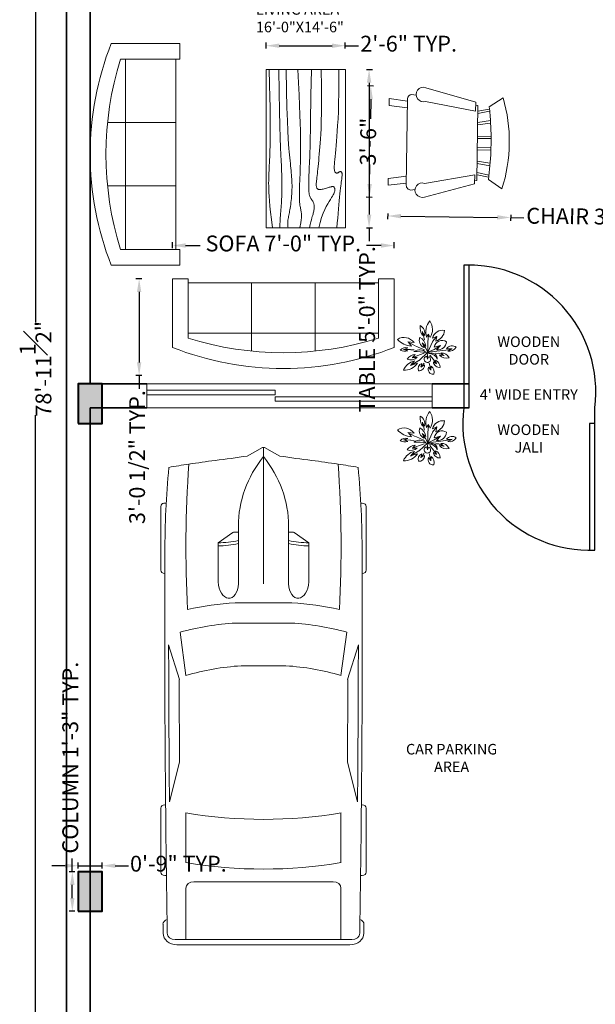
# Model space of a CAD drawing. Units: inches. Extents: x 2845 to 3575, y 808 to 1996.
# Tile 2 of 6: x 2955 to 3173, y 1215 to 1588. Entities that reach past the tile are written whole.
import ezdxf

# ---------------------------------------------------------------- set-up
doc = ezdxf.new("R2010")
doc.units = ezdxf.units.IN
for name, color, linetype, lineweight in [('A-ANNO-DIMS', 2, 'Continuous', 18), ('A-ANNO-TEXT', 7, 'Continuous', 18), ('A-AREA-IDEN', 7, 'Continuous', 18), ('A-COLS', 7, 'Continuous', 40), ('A-DOOR', 34, 'Continuous', 25), ('A-FURN', 30, 'Continuous', 18), ('A-GLAZ', 4, 'Continuous', 18), ('A-WALL', 1, 'Continuous', 35), ('C-PRKG-VEHI', 8, 'Continuous', 13), ('L-PLNT', 3, 'Continuous', 13)]:
    doc.layers.add(name, color=color, linetype=linetype, lineweight=lineweight)
doc.styles.get("Standard").update_dxf_attribs({"font": 'arial.ttf'})
doc.dimstyles.new('ISO-25', dxfattribs={"dimtxt": 6, "dimasz": 5, "dimexe": 1.25, "dimexo": 0.625, "dimtad": 0, "dimlunit": 4, "dimtxsty": 'Standard', "dimcen": 2.5, "dimclrd": 1, "dimclre": 1, "dimclrt": 1, "dimadec": 0, "dimazin": 0, "dimtfac": 1, "dimtmove": 0, "dimatfit": 3, "dimfxl": 1, "dimfxlon": 1, "dimfrac": 1, "dimarcsym": 0})

# ---------------------------------------------------------------- blocks, each defined once
blk = doc.blocks.new('Sofa - Roundback 7 ft.')
for p, q in [((-12.00002, -32.4421), (-12.00003, -6.5971)), ((11.99997, -32.4421), (11.99998, -6.5971)), ((-36.000027, -34), (-36.000027, -11.4696)), ((-35.999844, -13.3819), (35.9998, -13.3819)), ((35.99998, -34), (35.99998, -11.4696)), ((-36.000027, -32.4421), (35.99998, -32.4421))]:
    blk.add_line(p, q)
for points in [[(-36.000027, -34), (-42.000027, -34), (-42.000027, -8)], [(41.99998, -8), (41.99998, -34), (35.99998, -34)]]:
    blk.add_lwpolyline(points)
for centre, radius, start, end in [((0, -114.25), 114.25, 68.43141, 111.5686), ((-0.00001, -127.1968), 121.1968, 72.72033, 107.2797)]:
    blk.add_arc(centre, radius, start, end)
blk = doc.blocks.new('Table - Rectangular Woodgrain 60 x 30 in.')
for p, q in [((0, 0), (0, -30)), ((60, 0), (0, 0)), ((60, -30), (60, 0)), ((0, -30), (60, -30))]:
    blk.add_line(p, q)
for points in [[(0, -2.4), (4.8155, -2.418), (9.0302, -2.4688), (12.709, -2.5477), (15.9167, -2.65), (18.7181, -2.7711), (21.1781, -2.9063), (23.3616, -3.0508), (25.3333, -3.2), (27.1477, -3.3495), (28.8172, -3.4958), (30.3437, -3.636), (31.7291, -3.7667), (32.9756, -3.8849), (34.0849, -3.9875), (35.059, -4.0714), (35.9, -4.1334), (36.6114, -4.1711), (37.2041, -4.1854), (37.6906, -4.1779), (38.0833, -4.15), (38.3948, -4.1034), (38.6375, -4.0396), (38.8239, -3.9602), (38.9666, -3.8667), (39.0764, -3.7608), (39.1573, -3.6448), (39.2116, -3.521), (39.2416, -3.3917), (39.2498, -3.2593), (39.2385, -3.1261), (39.21, -2.9944), (39.1666, -2.8667), (39.111, -2.7447), (39.0468, -2.6281), (38.978, -2.5163), (38.9083, -2.4083), (38.8418, -2.3035), (38.7823, -2.201), (38.7337, -2.1001), (38.7, -2), (38.6844, -1.9003), (38.6875, -1.8021), (38.7094, -1.707), (38.75, -1.6167), (38.8094, -1.5326), (38.8875, -1.4563), (38.9844, -1.3893), (39.1, -1.3333), (39.2351, -1.2896), (39.3937, -1.2583), (39.5804, -1.2396), (39.8, -1.2333), (40.057, -1.2396), (40.3562, -1.2583), (40.7023, -1.2896), (41.1, -1.3333), (41.5547, -1.3895), (42.0755, -1.4573), (42.6721, -1.5361), (43.3542, -1.625), (44.1316, -1.7233), (45.014, -1.8302), (46.0114, -1.9449), (47.1333, -2.0667), (48.3862, -2.1947), (49.7625, -2.3281), (51.2513, -2.4663), (52.8416, -2.6083), (54.5226, -2.7535), (56.2833, -2.9011), (58.1127, -3.0501), (60, -3.2)], [(0, -9.2), (6.5759, -9.0858), (11.9385, -9.0365), (16.2527, -9.0418), (19.6833, -9.0917), (22.3952, -9.1759), (24.5531, -9.2844), (26.322, -9.4069), (27.8666, -9.5333), (29.3241, -9.6553), (30.7203, -9.7719), (32.0532, -9.8837), (33.3208, -9.9917), (34.5213, -10.0965), (35.6526, -10.199), (36.7128, -10.2999), (37.7, -10.4), (38.6129, -10.4996), (39.4531, -10.5969), (40.223, -10.6895), (40.925, -10.775), (41.5613, -10.8512), (42.1344, -10.9156), (42.6465, -10.966), (43.1, -11), (43.4976, -11.0158), (43.8437, -11.0136), (44.143, -10.9942), (44.4, -10.9583), (44.6195, -10.9069), (44.8062, -10.8406), (44.9648, -10.7603), (45.1, -10.6667), (45.2155, -10.5598), (45.3114, -10.4365), (45.3871, -10.2929), (45.4416, -10.125), (45.4743, -9.929), (45.4844, -9.7011), (45.4709, -9.4371), (45.4333, -9.1333), (45.3716, -8.7883), (45.2896, -8.4104), (45.1919, -8.0107), (45.0833, -7.6), (44.9685, -7.1893), (44.8521, -6.7896), (44.7388, -6.4117), (44.6333, -6.0667), (44.54, -5.7628), (44.4614, -5.4979), (44.4001, -5.2675), (44.3583, -5.0667), (44.3384, -4.8909), (44.3427, -4.7354), (44.3736, -4.5956), (44.4333, -4.4667), (44.5236, -4.3453), (44.6427, -4.2333), (44.7884, -4.1339), (44.9583, -4.05), (45.1501, -3.9849), (45.3614, -3.9417), (45.59, -3.9234), (45.8333, -3.9333), (46.0915, -3.9749), (46.3734, -4.0531), (46.6906, -4.1736), (47.0542, -4.3417), (47.4756, -4.5629), (47.9661, -4.8427), (48.5372, -5.1866), (49.2, -5.6), (49.9676, -6.0844), (50.8594, -6.625), (51.8965, -7.2031), (53.1, -7.8), (54.491, -8.3969), (56.0906, -8.975), (57.9199, -9.5156), (60, -10)], [(0, -12.8), (5.1847, -12.9322), (9.6213, -13.0323), (13.3963, -13.1059), (16.5958, -13.1583), (19.3063, -13.1952), (21.614, -13.2219), (23.6054, -13.2439), (25.3666, -13.2667), (26.9728, -13.2947), (28.4531, -13.3281), (29.8256, -13.3663), (31.1083, -13.4083), (32.3191, -13.4535), (33.476, -13.501), (34.597, -13.5501), (35.7, -13.6), (36.7984, -13.6497), (37.8875, -13.6979), (38.9578, -13.743), (40, -13.7833), (41.0047, -13.8174), (41.9625, -13.8438), (42.864, -13.8607), (43.7, -13.8667), (44.4631, -13.8604), (45.1552, -13.8417), (45.7801, -13.8104), (46.3416, -13.7667), (46.8439, -13.7104), (47.2906, -13.6417), (47.6858, -13.5604), (48.0333, -13.4667), (48.3375, -13.3608), (48.6042, -13.2448), (48.8396, -13.121), (49.05, -12.9917), (49.2417, -12.8593), (49.4208, -12.7261), (49.5937, -12.5944), (49.7667, -12.4667), (49.9452, -12.3451), (50.1323, -12.2313), (50.3303, -12.1268), (50.5416, -12.0333), (50.7686, -11.9524), (51.0135, -11.8854), (51.2788, -11.8341), (51.5666, -11.8), (51.8785, -11.7843), (52.2116, -11.7865), (52.562, -11.8059), (52.926, -11.8417), (53.2998, -11.8931), (53.6795, -11.9594), (54.0614, -12.0397), (54.4416, -12.1333), (54.8223, -12.2401), (55.2293, -12.3625), (55.6942, -12.5037), (56.2489, -12.6667), (56.9251, -12.8547), (57.7545, -13.0708), (58.7689, -13.3182), (60, -13.6)], [(0, -18), (5.124, -17.7273), (9.6609, -17.5057), (13.6705, -17.3303), (17.2125, -17.1958), (20.3467, -17.0973), (23.1328, -17.0297), (25.6307, -16.9878), (27.9, -16.9667), (29.9928, -16.9617), (31.9302, -16.9703), (33.7254, -16.9907), (35.3917, -17.0208), (36.9423, -17.0588), (38.3906, -17.1026), (39.7499, -17.1503), (41.0333, -17.2), (42.2519, -17.2496), (43.4073, -17.2969), (44.4986, -17.3395), (45.525, -17.375), (46.4858, -17.4012), (47.3802, -17.4156), (48.2074, -17.416), (48.9667, -17.4), (49.6583, -17.3662), (50.2872, -17.3167), (50.8595, -17.2547), (51.3812, -17.1833), (51.8584, -17.1057), (52.2971, -17.025), (52.7034, -16.9443), (53.0833, -16.8667), (53.443, -16.7951), (53.789, -16.7313), (54.128, -16.6768), (54.4666, -16.6334), (54.8115, -16.6024), (55.1693, -16.5854), (55.5465, -16.5841), (55.95, -16.6), (56.3828, -16.6337), (56.8346, -16.6823), (57.2915, -16.7418), (57.7396, -16.8084), (58.165, -16.878), (58.5539, -16.9469), (58.8924, -17.0111), (59.1666, -17.0667), (59.3679, -17.1107), (59.5078, -17.1438), (59.6032, -17.1675), (59.6708, -17.1833), (59.7275, -17.193), (59.7901, -17.1979), (59.8753, -17.1998), (60, -17.2)], [(0, -22.4), (8.0098, -22.2501), (14.4094, -22.1011), (19.4168, -21.9535), (23.25, -21.8083), (26.1269, -21.6663), (28.2656, -21.5281), (29.884, -21.3947), (31.2, -21.2667), (32.3967, -21.1448), (33.5172, -21.0292), (34.5697, -20.9198), (35.5625, -20.8167), (36.5037, -20.7198), (37.4015, -20.6292), (38.2642, -20.5448), (39.1, -20.4667), (39.9164, -20.3951), (40.7187, -20.3313), (41.5117, -20.2768), (42.3, -20.2333), (43.0883, -20.2024), (43.8812, -20.1854), (44.6836, -20.1841), (45.5, -20.2), (46.3328, -20.234), (47.1747, -20.2844), (48.0163, -20.3488), (48.8479, -20.425), (49.66, -20.5106), (50.4429, -20.6031), (51.1872, -20.7004), (51.8833, -20.8), (52.5246, -20.8999), (53.1166, -20.9995), (53.6681, -21.0983), (54.1875, -21.1958), (54.6834, -21.2919), (55.1646, -21.3859), (55.6394, -21.4777), (56.1167, -21.5667), (56.6028, -21.6515), (57.0961, -21.7266), (57.5929, -21.7852), (58.0896, -21.8208), (58.5823, -21.8268), (59.0674, -21.7964), (59.5412, -21.723), (60, -21.6)], [(0, -25.2), (8.6355, -25.0504), (15.7026, -24.9031), (21.4049, -24.7606), (25.9458, -24.625), (29.529, -24.4988), (32.3578, -24.3844), (34.6359, -24.284), (36.5667, -24.2), (38.3213, -24.1341), (39.9417, -24.0854), (41.437, -24.0523), (42.8167, -24.0333), (44.0901, -24.0268), (45.2667, -24.0313), (46.3557, -24.0451), (47.3667, -24.0667), (48.309, -24.0947), (49.1928, -24.1287), (50.0284, -24.168), (50.826, -24.2125), (51.5959, -24.2617), (52.3483, -24.3151), (53.0935, -24.3725), (53.8417, -24.4334), (54.6009, -24.497), (55.3699, -24.561), (56.1454, -24.6226), (56.9239, -24.6792), (57.7021, -24.7279), (58.4764, -24.7662), (59.2435, -24.7911), (60, -24.8)], [(0, -28.8), (5.6867, -28.6681), (10.45, -28.5698), (14.407, -28.5012), (17.675, -28.4584), (20.3711, -28.4374), (22.6125, -28.4344), (24.5164, -28.4455), (26.2, -28.4667), (27.762, -28.4947), (29.2276, -28.5281), (30.6033, -28.5663), (31.8958, -28.6084), (33.1118, -28.6535), (34.2578, -28.7011), (35.3405, -28.7501), (36.3666, -28.8), (37.3443, -28.8497), (38.288, -28.8974), (39.2137, -28.9412), (40.1375, -28.9792), (41.0753, -29.0093), (42.0432, -29.0297), (43.0572, -29.0384), (44.1333, -29.0333), (45.2936, -29.0114), (46.5843, -28.9641), (48.0579, -28.8816), (49.7666, -28.7542), (51.7629, -28.5721), (54.0989, -28.3255), (56.8272, -28.0048), (60, -27.6)]]:
    blk.add_lwpolyline(points)
blk = doc.blocks.new('Chair - Rocking')
for p, q in [((-8, -4.5), (-10, -1.5)), ((8, -4.5), (10, -1.5)), ((-4.5, -7), (-4.96674, -4.19951)), ((-4, -7), (-4.40532, -4.16272)), ((-1.5, -4.05012), (-1.5, -7)), ((-1, -7), (-1, -4.05012)), ((1, -7), (1, -4.04655)), ((1.5, -4.05012), (1.5, -7)), ((4, -7), (4.40187, -4.18694)), ((4.5, -7), (4.96761, -4.19437)), ((-7.5, -4.5), (-7, -7)), ((-6.5, -7), (-7.02225, -4.43)), ((6.5, -7), (7, -4.4057)), ((7.5, -4.5), (7, -7)), ((-9, -7.5), (-12, -18.49999)), ((-7, -7.5), (-9, -7.5)), ((-9, -18.49999), (-7, -7.5)), ((-8.23428, -6.99939), (-8.3093, -7.47958)), ((-8.23041, -7), (8.23915, -7)), ((7, -7.5), (9, -7.5)), ((9, -18.49999), (7, -7.5)), ((8.31071, -7.48854), (8.23449, -7.00073)), ((9, -7.5), (12, -18.49999)), ((-10.36644, -20.64523), (-10.5, -21.49999)), ((10.5, -21.49999), (10.3575, -20.58798)), ((-9, -22.49999), (-9.5, -26.49999)), ((0, -22.49999), (-9.5, -22.49999)), ((-8, -26.49999), (-7.5, -22.49999)), ((0, -22.49999), (9.5, -22.49999)), ((8, -26.49999), (7.5, -22.49999)), ((9, -22.49999), (9.5, -26.49999)), ((-9.5, -26.49999), (-8, -26.49999)), ((9.5, -26.49999), (8, -26.49999))]:
    blk.add_line(p, q)
for centre, radius, start, end in [((0, -34.08333), 34.08333, 72.93847, 107.0615), ((0, -68.25004), 64.25, 93.92211, 97.15267), ((0, -68.25004), 64.25, 82.84733, 93.92211), ((-10.5, -18.99999), 1.58114, 161.5651, 18.43495), ((10.5, -18.99999), 1.58114, 161.5651, 18.43495), ((-9.5, -21.49999), 1, 180, 270), ((9.5, -21.49999), 1, 270, 0)]:
    blk.add_arc(centre, radius, start, end)
blk = doc.blocks.new('z_109')
for p, q in [((-94, 294), (-122, 396)), ((-121, 393), (-119, 324)), ((-120, 377), (-82, 322)), ((-392, 202), (-278, 190)), ((-254, 128), (-392, 202)), ((-390, 202), (-327, 125)), ((-61, 92), (-128, 186)), ((-85, 244), (-94, 293)), ((-5, 350), (-42, 295)), ((-20, 11), (-18, 230)), ((-20, 11), (65, 205)), ((-14, 234), (-5, 350)), ((-5, 350), (24, 284)), ((65, 209), (150, 307)), ((65, 205), (65, 205)), ((150, 307), (68, 272)), ((129, 216), (150, 307)), ((150, 307), (129, 216)), ((-342, 60), (-472, 63)), ((-467, 63), (-392, 90)), ((-463, 64), (-392, 37)), ((-276, 53), (-338, 57)), ((-84, 54), (-246, 125)), ((-20, 11), (-181, -143)), ((-126, 184), (-60, 125)), ((-120, 176), (-91, 98)), ((-20, 11), (-61, 92)), ((-20, 11), (-24, -65)), ((-20, 11), (102, 64)), ((-20, 11), (-14, 11)), ((-14, 11), (319, 50)), ((-14, 11), (-13, 13)), ((-13, 13), (13, -13)), ((217, 135), (101, 105)), ((102, 64), (217, 135)), ((217, 135), (145, 55)), ((319, 50), (434, 75)), ((429, 74), (333, 77)), ((428, 74), (353, 32)), ((-187, -143), (-345, -240)), ((-342, -238), (-269, -151)), ((-178, -41), (-313, -92)), ((-308, -90), (-254, -33)), ((-306, -89), (-217, -88)), ((-86, -8), (-178, -41)), ((-26, -113), (-45, -66)), ((-24, -65), (-28, -121)), ((-28, -117), (-2, -69)), ((16, -43), (88, -126)), ((141, -208), (84, -170)), ((87, -129), (140, -204)), ((122, -8), (193, -11)), ((140, -205), (123, -139)), ((176, -10), (285, -54)), ((283, -54), (196, -42)), ((273, -52), (222, -4)), ((-328, -230), (-213, -195)), ((-151, -267), (-81, -228)), ((-89, -192), (-150, -267)), ((-150, -266), (-131, -199)), ((34, -320), (-6, -268)), ((4, -192), (16, -238)), ((16, -238), (35, -326)), ((35, -327), (45, -249))]:
    blk.add_line(p, q)
for centre, radius, start, end in [((262, 393), 319, 140.563, 197.8988), ((-221, 433), 288, 328.6458, 34.5329), ((84, 468), 249, 170.3029, 215.3262), ((-235, 368), 160, 343.2534, 62.5239), ((256, 231), 192, 77.7318, 167.6805), ((55, 447), 242, 287.7269, 353.3689), ((-464, 59), 228, 35.1725, 122.5976), ((-304, 504), 380, 221.8384, 266.6027), ((-21, 239), 158, 161.4501, 243.415), ((-251, 115), 192, 2.9136, 65.0019), ((247, 86), 147, 55.2824, 172.6291), ((167, 217), 164, 262.2896, 356.2544), ((-434, -39), 136, 71.6414, 139.5892), ((-450, 225), 197, 243.5199, 287.2599), ((-173, -118), 175, 44.3837, 127.1057), ((-243, -1063), 1086, 79.6239, 91.8656), ((434, 8), 123, 51.1111, 145.9654), ((384, 175), 146, 257.8549, 330.7421), ((-198, -444), 302, 103.499, 156.8265), ((-246, -222), 190, 92.4489, 147.0817), ((-337, 52), 185, 248.0932, 310.529), ((-31, -123), 58.9, 103.4106, 268.148), ((-26, -123), 58.9, 262.5922, 66.6581), ((53, -110), 105, 354.7987, 111.9005), ((2, -181), 167, 21.6922, 85.2277), ((197, -160), 113, 185.1842, 278.9266), ((66, -276), 148, 1.4924, 67.3596), ((325, 60), 164, 218.6232, 288.4099), ((241, -149), 146, 21.4559, 97.3107), ((-455, -39), 287, 265.8156, 327.2626), ((-94, -301), 109, 109.8936, 199.3062), ((-186, -232), 105, 264.4232, 2.0221), ((80, -308), 95.1, 155.1092, 275.9038), ((-28, -354), 128, 337.3115, 55.0978)]:
    blk.add_arc(centre, radius, start, end)
blk = doc.blocks.new('*U21')
for p, q in [((21.1, 37.41), (21.1, 36.83)), ((46.55, 38.89), (22.35, 38.89)), ((47.8, 37.39), (47.8, 37.41)), ((135.45, 37.07), (135.45, 37.41)), ((136.7, 38.89), (160.9, 38.89)), ((162.15, 37.41), (162.15, 36.77)), ((87.99, 31.87), (74.76, 35.92)), ((134.31, 35.6), (119.29, 31.78)), ((70.03, 31.54), (86.41, 29.35)), ((186.47, -33.5), (186.47, 33.5)), ((188.4, -32.76), (188.4, 32.76)), ((138.42, 29.35), (157.25, 29.35)), ((164.52, 26.39), (164.52, -26.39)), ((186.47, 29.35), (167.01, 29.35)), ((32.27, 11.63), (36.13, 17.17)), ((36.13, 17.17), (50.94, 17.17)), ((29.77, 9.51), (51.68, 9.51)), ((32.12, 9.51), (32.12, 11.15)), ((58.92, -10.77), (58.92, 10.77)), ((66.55, -10.53), (66.55, 10.53)), ((82.74, 8.5), (82.74, -8.5)), ((186.47, -10.53), (186.47, 10.53)), ((3.27, 6.13), (0.1, 0.41)), ((0, 0), (51.68, 0)), ((0.1, -0.41), (3.27, -6.13)), ((29.77, -9.51), (51.68, -9.51)), ((32.12, -9.51), (32.12, -11.15)), ((32.27, -11.63), (36.13, -17.17)), ((36.13, -17.17), (50.94, -17.17)), ((86.41, -29.35), (70.03, -31.54)), ((157.25, -29.35), (138.42, -29.35)), ((167.01, -29.35), (186.47, -29.35)), ((87.99, -31.87), (74.76, -35.92)), ((134.31, -35.6), (119.29, -31.78)), ((21.1, -37.41), (21.1, -36.83)), ((135.45, -37.07), (135.45, -37.41)), ((162.15, -37.41), (162.15, -36.77)), ((46.55, -38.89), (22.35, -38.89)), ((47.8, -37.39), (47.8, -37.41)), ((136.7, -38.89), (160.9, -38.89))]:
    blk.add_line(p, q)
for centre, major_axis, ratio, start_param, end_param in [((41.19, -490.86), (0, 528.23), 0.842304, 0.00281, 0.075598), ((22.35, 37.41), (0, -1.48), 0.842304, 3.141593, 4.712389), ((64.48, -10555.62), (0, 10593.03), 0.842304, -0.013397, 0.002797), ((46.55, 37.41), (0, 1.48), 0.842304, -1.570796, 0), ((136.7, 37.41), (0, -1.48), 0.842304, 3.141593, 4.712389), ((160.9, 37.41), (0, 1.48), 0.842304, -1.570796, 0), ((180.63, 35.84), (0, 2.22), 0.842304, -0.013017, 1.249894), ((64.48, -10556.36), (0, 10595.31), 0.842304, -0.013397, -0.013017), ((183.98, 32.76), (0, -5.25), 0.842304, 1.570796, 3.128196), ((266.03, -27.52), (0, 313.31), 0.842304, 1.367076, 1.39176), ((64.48, -10555.62), (0, -10591.55), 0.842304, 3.133765, 3.140441), ((183.98, 33.5), (0, -2.96), 0.842304, 1.570796, 3.128196), ((135.29, 5.39), (0, 81.77), 0.842304, 1.245306, 1.50788), ((95.79, -3666.35), (0, -3698.24), 0.842304, 3.134049, 3.144098), ((259.18, -27.52), (0, -305.3), 0.842304, 4.528606, 4.561838), ((37.47, -593.96), (0, -623.33), 0.842304, 3.096046, 3.200911), ((134.4, 5.39), (0, -89.78), 0.842304, 4.449482, 4.652344), ((149.6, 2.8), (0, -79.58), 0.842304, 4.372215, 4.640744), ((17.08, 0), (0, 147.02), 0.842304, 4.511394, 4.913384), ((35.91, 0), (0, 147.02), 0.842304, 4.511394, 4.913384), ((167.01, 26.39), (0, 2.96), 0.842304, 0, 1.570796), ((-204.49, 52.4), (0, -250.96), 0.842304, 1.385369, 1.434372), ((13.04, 17.01), (0, 27.42), 0.842304, 4.435146, 4.718221), ((14.2, 17.01), (0, 27.42), 0.842304, 4.435146, 4.718221), ((50.79, 13.34), (6.34, -0.36), 0.603834, -1.395552, 1.581315), ((32.75, 11.15), (0, 0.74), 0.842304, 0.879714, 1.570796), ((29.77, -46.66), (0, 56.17), 0.842304, 0, 0.590319), ((0.62, 0), (0, -0.74), 0.842304, 4.131459, 5.293319), ((29.77, 46.66), (0, 56.17), 0.842304, 2.551274, 3.141593), ((-204.49, -52.4), (0, 250.96), 0.842304, -1.434372, -1.385369), ((32.75, -11.15), (0, -0.74), 0.842304, 4.712389, 5.403472), ((13.04, -17.01), (0, -27.42), 0.842304, 1.564964, 1.848039), ((14.2, -17.01), (0, -27.42), 0.842304, 1.564964, 1.848039), ((134.4, -5.39), (0, -89.78), 0.842304, -1.510751, -1.307889), ((135.29, -5.39), (0, -81.77), 0.842304, -1.50788, -1.245306), ((149.6, -2.8), (0, -79.58), 0.842304, -1.499151, -1.230623), ((259.18, 27.52), (0, 305.3), 0.842304, 1.721348, 1.754579), ((266.03, 27.52), (0, 313.31), 0.842304, 1.749832, 1.774517), ((37.47, 593.96), (0, -623.33), 0.842304, -0.059319, 0.045547), ((167.01, -26.39), (0, -2.96), 0.842304, 4.712389, 6.283185), ((95.79, 3666.35), (0, -3698.24), 0.842304, -0.002505, 0.007544), ((183.98, -33.5), (0, 2.96), 0.842304, 3.15499, 4.712389), ((183.98, -32.76), (0, -5.25), 0.842304, 0.013397, 1.570796), ((41.19, 490.86), (0, -528.23), 0.842304, -0.075598, -0.00281), ((64.48, 10555.62), (0, 10593.03), 0.842304, 3.138796, 3.15499), ((64.48, 10555.62), (0, -10591.55), 0.842304, 0.001152, 0.007828), ((180.63, -35.84), (0, -2.22), 0.842304, -1.249894, 0.013017), ((22.35, -37.41), (0, 1.48), 0.842304, 1.570796, 3.141593), ((46.55, -37.41), (0, -1.48), 0.842304, 0, 1.570796), ((136.7, -37.41), (0, -1.48), 0.842304, -1.570796, 0), ((160.9, -37.41), (0, 1.48), 0.842304, 3.141593, 4.712389), ((64.48, 10556.36), (0, 10595.31), 0.842304, 3.15461, 3.15499)]:
    blk.add_ellipse(centre, major_axis=major_axis, ratio=ratio, start_param=start_param, end_param=end_param)
at = {"extrusion": (0, 0, -1)}
blk.add_ellipse((50.79, -13.34), major_axis=(6.34, 0.36), ratio=0.603834, start_param=-1.395552, end_param=1.581315, dxfattribs=at)
blk = doc.blocks.new('*D30')
at = {"layer": 'A-ANNO-DIMS', "color": 0, "lineweight": -2, "transparency": 16777216}
for p, q in [((2961.94, 1929.67), (2959.69, 1929.67)), ((2960.94, 1924.67), (2960.94, 1473.45)), ((2960.94, 987.17), (2960.94, 1438.39)), ((2961.94, 982.17), (2959.69, 982.17))]:
    blk.add_line(p, q, dxfattribs=at)
at = {"layer": 'A-ANNO-DIMS', "color": 0, "transparency": 16777216}
for points in [[(2960.11, 1924.67), (2961.77, 1924.67), (2960.94, 1929.67)], [(2960.11, 987.17), (2961.77, 987.17), (2960.94, 982.17)]]:
    blk.add_solid(points, dxfattribs=at)
at = {"layer": 'Defpoints', "color": 0, "transparency": 16777216}
for p in [(2972.62, 1929.67), (2960.94, 982.17), (2972.62, 982.17)]:
    blk.add_point(p, dxfattribs=at)
at = {"layer": 'A-ANNO-DIMS', "color": 0, "transparency": 16777216, "insert": (2960.94, 1455.92), "char_height": 6, "attachment_point": 5, "rotation": 90}
blk.add_mtext('78\'-11{\\H1x;\\S1#2;}"', dxfattribs=at)
blk = doc.blocks.new('COL-9x15')
h = blk.add_hatch(color=256)
h.dxf.hatch_style = 1
h.paths.add_polyline_path([(0, 0), (9, 0), (9, 15), (0, 15)])
blk.add_lwpolyline([(0, 0), (9, 0), (9, 15), (0, 15)], close=True)
blk = doc.blocks.new('*D44')
at = {"layer": 'A-ANNO-DIMS', "color": 1, "lineweight": -2, "transparency": 16777216}
for p, q in [((2974.87, 1265.42), (2974.87, 1270.42)), ((2975.87, 1265.42), (2973.62, 1265.42)), ((2974.87, 1255.42), (2974.87, 1260.42)), ((2975.87, 1250.42), (2973.62, 1250.42))]:
    blk.add_line(p, q, dxfattribs=at)
at = {"layer": 'A-ANNO-DIMS', "color": 1, "transparency": 16777216}
for points in [[(2974.03, 1260.42), (2975.7, 1260.42), (2974.87, 1265.42)], [(2974.03, 1255.42), (2975.7, 1255.42), (2974.87, 1250.42)]]:
    blk.add_solid(points, dxfattribs=at)
at = {"layer": 'Defpoints', "color": 0, "transparency": 16777216}
for p in [(2974.87, 1265.42), (2977.12, 1265.42), (2977.12, 1250.42)]:
    blk.add_point(p, dxfattribs=at)
at = {"layer": 'A-ANNO-DIMS', "color": 1, "transparency": 16777216, "insert": (2974.87, 1308.62), "char_height": 6, "attachment_point": 5, "rotation": 90}
blk.add_mtext('COLUMN 1\'-3" TYP.', dxfattribs=at)
blk = doc.blocks.new('*D45')
at = {"layer": 'A-ANNO-DIMS', "color": 1, "lineweight": -2, "transparency": 16777216}
for p, q in [((2977.12, 1266.67), (2977.12, 1268.92)), ((2986.12, 1266.67), (2986.12, 1268.92)), ((2972.12, 1267.67), (2967.12, 1267.67)), ((2977.12, 1267.67), (2986.12, 1267.67)), ((2991.12, 1267.67), (2996.12, 1267.67))]:
    blk.add_line(p, q, dxfattribs=at)
at = {"layer": 'A-ANNO-DIMS', "color": 1, "transparency": 16777216}
for points in [[(2972.12, 1268.5), (2972.12, 1266.83), (2977.12, 1267.67)], [(2991.12, 1268.5), (2991.12, 1266.83), (2986.12, 1267.67)]]:
    blk.add_solid(points, dxfattribs=at)
at = {"layer": 'Defpoints', "color": 0, "transparency": 16777216}
for p in [(2977.12, 1265.42), (2986.12, 1267.67), (2986.12, 1265.42)]:
    blk.add_point(p, dxfattribs=at)
at = {"layer": 'A-ANNO-DIMS', "color": 1, "transparency": 16777216, "insert": (3015.03, 1267.67), "char_height": 6, "attachment_point": 5}
blk.add_mtext('0\'-9" TYP.', dxfattribs=at)
blk = doc.blocks.new('*D52')
at = {"layer": 'A-ANNO-DIMS', "color": 1, "lineweight": -2, "transparency": 16777216}
for p, q in [((3012.78, 1501.62), (3012.78, 1503.87)), ((3096.78, 1501.62), (3096.78, 1503.87)), ((3017.78, 1502.62), (3023.31, 1502.62)), ((3091.78, 1502.62), (3086.25, 1502.62))]:
    blk.add_line(p, q, dxfattribs=at)
at = {"layer": 'A-ANNO-DIMS', "color": 1, "transparency": 16777216}
for points in [[(3017.78, 1503.46), (3017.78, 1501.79), (3012.78, 1502.62)], [(3091.78, 1503.46), (3091.78, 1501.79), (3096.78, 1502.62)]]:
    blk.add_solid(points, dxfattribs=at)
at = {"layer": 'Defpoints', "color": 0, "transparency": 16777216}
for p in [(3012.78, 1502.62), (3012.78, 1490.02), (3096.78, 1490.02)]:
    blk.add_point(p, dxfattribs=at)
at = {"layer": 'A-ANNO-DIMS', "color": 1, "transparency": 16777216, "insert": (3054.78, 1502.62), "char_height": 6, "attachment_point": 5}
blk.add_mtext('SOFA 7\'-0" TYP.', dxfattribs=at)
blk = doc.blocks.new('*D53')
at = {"layer": 'A-ANNO-DIMS', "color": 1, "lineweight": -2, "transparency": 16777216}
for p, q in [((3001.18, 1490.02), (2998.93, 1490.02)), ((3000.18, 1485.02), (3000.18, 1458.36)), ((3001.18, 1453.36), (2998.93, 1453.36)), ((3000.18, 1453.36), (3000.18, 1448.36))]:
    blk.add_line(p, q, dxfattribs=at)
at = {"layer": 'A-ANNO-DIMS', "color": 1, "transparency": 16777216}
for points in [[(2999.35, 1485.02), (3001.01, 1485.02), (3000.18, 1490.02)], [(2999.35, 1458.36), (3001.01, 1458.36), (3000.18, 1453.36)]]:
    blk.add_solid(points, dxfattribs=at)
at = {"layer": 'Defpoints', "color": 0, "transparency": 16777216}
for p in [(3012.78, 1490.02), (3000.18, 1453.36), (3012.78, 1453.36)]:
    blk.add_point(p, dxfattribs=at)
at = {"layer": 'A-ANNO-DIMS', "color": 1, "transparency": 16777216, "insert": (3000.18, 1422.46), "char_height": 6, "attachment_point": 5, "rotation": 90}
blk.add_mtext('3\'-0 1/2" TYP.', dxfattribs=at)
blk = doc.blocks.new('*D54')
at = {"layer": 'A-ANNO-DIMS', "color": 1, "lineweight": -2, "transparency": 16777216}
for p, q in [((3094.31, 1514.81), (3094.28, 1512.56)), ((3099.3, 1513.75), (3135.88, 1513.29)), ((3140.89, 1514.23), (3140.86, 1511.98)), ((3140.88, 1513.23), (3145.88, 1513.16))]:
    blk.add_line(p, q, dxfattribs=at)
at = {"layer": 'A-ANNO-DIMS', "color": 1, "transparency": 16777216}
for points in [[(3099.31, 1514.58), (3099.29, 1512.91), (3094.3, 1513.81)], [(3135.89, 1514.12), (3135.87, 1512.45), (3140.88, 1513.23)]]:
    blk.add_solid(points, dxfattribs=at)
at = {"layer": 'Defpoints', "color": 0, "transparency": 16777216}
for p in [(3094.39, 1520.79), (3140.96, 1520.21), (3140.88, 1513.23)]:
    blk.add_point(p, dxfattribs=at)
at = {"layer": 'A-ANNO-DIMS', "color": 1, "transparency": 16777216, "insert": (3177.96, 1512.76), "char_height": 6, "attachment_point": 5, "rotation": 359.2832}
blk.add_mtext('CHAIR 3\'-10 1/2"', dxfattribs=at)
blk = doc.blocks.new('*D55')
at = {"layer": 'A-ANNO-DIMS', "color": 1, "lineweight": -2, "transparency": 16777216}
for p, q in [((3088.93, 1563.02), (3086.68, 1563.05)), ((3087.87, 1558.03), (3087.77, 1550.56)), ((3087.46, 1525.88), (3087.56, 1533.36)), ((3088.4, 1520.87), (3086.15, 1520.9))]:
    blk.add_line(p, q, dxfattribs=at)
at = {"layer": 'A-ANNO-DIMS', "color": 1, "transparency": 16777216}
for points in [[(3087.03, 1558.04), (3088.7, 1558.02), (3087.93, 1563.03)], [(3086.63, 1525.89), (3088.3, 1525.87), (3087.4, 1520.88)]]:
    blk.add_solid(points, dxfattribs=at)
at = {"layer": 'Defpoints', "color": 0, "transparency": 16777216}
for p in [(3094.91, 1562.95), (3087.4, 1520.88), (3094.39, 1520.79)]:
    blk.add_point(p, dxfattribs=at)
at = {"layer": 'A-ANNO-DIMS', "color": 1, "transparency": 16777216, "insert": (3087.66, 1541.96), "char_height": 6, "attachment_point": 5, "rotation": 89.2832}
blk.add_mtext('3\'-6"', dxfattribs=at)
blk = doc.blocks.new('*D60')
at = {"layer": 'A-ANNO-DIMS', "color": 1, "lineweight": -2, "transparency": 16777216}
for p, q in [((3086.26, 1569.31), (3088.51, 1569.31)), ((3087.26, 1564.31), (3087.26, 1514.31)), ((3086.26, 1509.31), (3088.51, 1509.31)), ((3087.26, 1509.31), (3087.26, 1504.31))]:
    blk.add_line(p, q, dxfattribs=at)
at = {"layer": 'A-ANNO-DIMS', "color": 1, "transparency": 16777216}
for points in [[(3086.43, 1564.31), (3088.1, 1564.31), (3087.26, 1569.31)], [(3086.43, 1514.31), (3088.1, 1514.31), (3087.26, 1509.31)]]:
    blk.add_solid(points, dxfattribs=at)
at = {"layer": 'Defpoints', "color": 0, "transparency": 16777216}
for p in [(3078.26, 1569.31), (3078.26, 1509.31), (3087.26, 1509.31)]:
    blk.add_point(p, dxfattribs=at)
at = {"layer": 'A-ANNO-DIMS', "color": 1, "transparency": 16777216, "insert": (3087.26, 1470.89), "char_height": 6, "attachment_point": 5, "rotation": 90}
blk.add_mtext('TABLE 5\'-0" TYP.', dxfattribs=at)
blk = doc.blocks.new('*D61')
at = {"layer": 'A-ANNO-DIMS', "color": 1, "lineweight": -2, "transparency": 16777216}
for p, q in [((3048.26, 1577.31), (3048.26, 1579.56)), ((3053.26, 1578.31), (3073.26, 1578.31)), ((3078.26, 1577.31), (3078.26, 1579.56)), ((3078.26, 1578.31), (3083.26, 1578.31))]:
    blk.add_line(p, q, dxfattribs=at)
at = {"layer": 'A-ANNO-DIMS', "color": 1, "transparency": 16777216}
for points in [[(3053.26, 1579.15), (3053.26, 1577.48), (3048.26, 1578.31)], [(3073.26, 1579.15), (3073.26, 1577.48), (3078.26, 1578.31)]]:
    blk.add_solid(points, dxfattribs=at)
at = {"layer": 'Defpoints', "color": 0, "transparency": 16777216}
for p in [(3078.26, 1578.31), (3048.26, 1569.31), (3078.26, 1569.31)]:
    blk.add_point(p, dxfattribs=at)
at = {"layer": 'A-ANNO-DIMS', "color": 1, "transparency": 16777216, "insert": (3102.23, 1578.31), "char_height": 6, "attachment_point": 5}
blk.add_mtext('2\'-6" TYP.', dxfattribs=at)
blk = doc.blocks.new('*D73')
at = {"layer": 'A-ANNO-DIMS', "color": 1, "lineweight": -2, "transparency": 16777216}
for p, q in [((2986.12, 844.33), (2986.12, 842.08)), ((2991.12, 843.33), (3069.97, 843.33)), ((3170.12, 843.33), (3091.26, 843.33)), ((3175.12, 844.33), (3175.12, 842.08))]:
    blk.add_line(p, q, dxfattribs=at)
at = {"layer": 'A-ANNO-DIMS', "color": 1, "transparency": 16777216}
for points in [[(2991.12, 844.17), (2991.12, 842.5), (2986.12, 843.33)], [(3170.12, 844.17), (3170.12, 842.5), (3175.12, 843.33)]]:
    blk.add_solid(points, dxfattribs=at)
at = {"layer": 'Defpoints', "color": 0, "transparency": 16777216}
for p in [(2986.12, 1250.42), (3175.12, 1252.17), (3175.12, 843.33)]:
    blk.add_point(p, dxfattribs=at)
at = {"layer": 'A-ANNO-DIMS', "color": 1, "transparency": 16777216, "insert": (3080.62, 843.33), "char_height": 6, "attachment_point": 5}
blk.add_mtext('15\'-9"', dxfattribs=at)
blk = doc.blocks.new('*D76')
at = {"layer": 'A-ANNO-DIMS', "color": 1, "lineweight": -2, "transparency": 16777216}
for p, q in [((3003.12, 844.33), (3003.12, 842.08)), ((3008.12, 843.33), (3048.52, 843.33)), ((3106.12, 843.33), (3065.72, 843.33)), ((3111.12, 844.33), (3111.12, 842.08))]:
    blk.add_line(p, q, dxfattribs=at)
at = {"layer": 'A-ANNO-DIMS', "color": 1, "transparency": 16777216}
for points in [[(3008.12, 844.17), (3008.12, 842.5), (3003.12, 843.33)], [(3106.12, 844.17), (3106.12, 842.5), (3111.12, 843.33)]]:
    blk.add_solid(points, dxfattribs=at)
at = {"layer": 'Defpoints', "color": 0, "transparency": 16777216}
for p in [(3003.12, 1441.17), (3111.12, 1441.17), (3111.12, 843.33)]:
    blk.add_point(p, dxfattribs=at)
at = {"layer": 'A-ANNO-DIMS', "color": 1, "transparency": 16777216, "insert": (3057.12, 843.33), "char_height": 6, "attachment_point": 5}
blk.add_mtext('9\'-0"', dxfattribs=at)

msp = doc.modelspace()

# ---------------------------------------------------------------- linework, layer by layer
at = {"layer": 'A-DOOR'}
for p, q in [((3123.116, 1495.173), (3123.116, 1441.173)), ((3125.116, 1450.173), (3125.116, 1495.173)), ((3127.116, 1495.173), (3125.116, 1495.173)), ((3125.116, 1450.173), (3123.116, 1450.173)), ((3125.116, 1441.173), (3125.116, 1450.173)), ((3172.739, 1435.173), (3172.739, 1441.173)), ((3170.739, 1435.173), (3170.739, 1387.173)), ((3172.739, 1435.173), (3170.739, 1435.173)), ((3172.739, 1387.173), (3172.739, 1435.173))]:
    msp.add_line(p, q, dxfattribs=at)
for centre, start, end in [((3125.116, 1447.173), 352.81924, 92.38802), ((3170.739, 1435.173), 172.81924, 272.38802)]:
    msp.add_arc(centre, 48, start, end, dxfattribs=at)
at = {"layer": 'A-GLAZ'}
for p, q in [((3003.116, 1450.173), (3003.116, 1441.173)), ((3003.116, 1450.173), (3111.116, 1450.173)), ((3003.116, 1450.173), (3100.239, 1450.173)), ((3003.116, 1447.798), (3051.677, 1447.798)), ((3051.677, 1447.798), (3051.677, 1446.065)), ((3111.116, 1450.173), (3111.116, 1441.173)), ((3051.677, 1446.065), (3003.116, 1446.065)), ((3051.677, 1443.622), (3051.677, 1445.358)), ((3051.677, 1445.358), (3111.116, 1445.358)), ((3111.116, 1443.622), (3051.677, 1443.622)), ((3003.116, 1441.173), (3111.116, 1441.173))]:
    msp.add_line(p, q, dxfattribs=at)
at = {"layer": 'A-WALL'}
for p, q in [((2972.616, 1798.173), (2972.616, 1143.734)), ((2981.616, 1624.173), (2981.616, 1450.173)), ((3003.116, 1450.173), (2981.616, 1450.173)), ((3125.116, 1450.173), (3111.116, 1450.173)), ((3003.116, 1441.173), (2981.616, 1441.173)), ((2981.616, 1441.173), (2981.616, 1143.734)), ((3125.116, 1441.173), (3111.116, 1441.173))]:
    msp.add_line(p, q, dxfattribs=at)

# ---------------------------------------------------------------- block references
at = {"layer": 'A-COLS'}
for p in [(2977.116, 1435.173), (2977.116, 1250.417)]:
    msp.add_blockref('COL-9x15', p, dxfattribs=at)
at = {"layer": 'A-FURN'}
for name, p, rotation in [('Sofa - Roundback 7 ft.', (2981.616, 1537.173), 90), ('Table - Rectangular Woodgrain 60 x 30 in.', (3078.263, 1569.315), 270), ('Sofa - Roundback 7 ft.', (3054.78, 1456.022), 180)]:
    msp.add_blockref(name, p, dxfattribs=dict(at, rotation=rotation))
at = {"layer": 'A-FURN', "xscale": 1.725193154276141, "yscale": 1.725193154276141, "zscale": 1.725193154276141, "rotation": 269.2831862631142}
msp.add_blockref('Chair - Rocking', (3140.364, 1541.299), dxfattribs=at)
at = {"layer": 'C-PRKG-VEHI', "rotation": 270}
msp.add_blockref('*U21', (3047.269, 1426.146), dxfattribs=at)
at = {"layer": 'L-PLNT', "xscale": 0.0202275909996564, "yscale": 0.0202275909996564, "zscale": 0.0202275909996564}
for p in [(3109.9, 1461.988), (3109.9, 1427.687)]:
    msp.add_blockref('z_109', p, dxfattribs=at)

# ---------------------------------------------------------------- texts
at = {"layer": 'A-ANNO-TEXT', "insert": (3125.116, 1468.173), "char_height": 4, "attachment_point": 1}
msp.add_mtext_dynamic_manual_height_columns("\\pxqc;WOODEN \\PDOOR\\P\\P4' WIDE ENTRY\\P\\PWOODEN \\PJALI", width=45.255, gutter_width=12.5, heights=[0], dxfattribs=at)
at = {"layer": 'A-AREA-IDEN', "char_height": 4, "attachment_point": 1}
for s, insert in [('LIVING AREA\\P16\'-0"X14\'-6"', (3044.406, 1594.068)), ('\\pxqc;CAR PARKING\\PAREA', (3095.883, 1313.812))]:
    msp.add_mtext_dynamic_manual_height_columns(s, width=45.255, gutter_width=12.5, heights=[0], dxfattribs=dict(at, insert=insert))

# ---------------------------------------------------------------- dimensions: what is measured, and where the dimension line sits
at = {"layer": 'A-ANNO-DIMS'}
for base, p1, p2, angle, override, picture, middle in [((2960.94, 982.173), (2972.616, 1929.673), (2972.616, 982.173), 90, {"dimclrd": 0, "dimclre": 0, "dimclrt": 0}, '*D30', (2960.94, 1455.923)), ((3087.4, 1520.882), (3094.914, 1562.947), (3094.387, 1520.795), 269.28319, {"dimdec": 1, "dimlfac": 1, "dimrnd": 0, "dimzin": 1, "dimdsep": 46, "dimlunit": 4, "dimfrac": 2}, '*D55', (3087.664, 1541.958))]:
    dim = msp.add_linear_dim(base=base, p1=p1, p2=p2, angle=angle, dimstyle='ISO-25', override=override, dxfattribs=at)
    dim.commit()
    dim.dimension.update_dxf_attribs({"geometry": picture, "text_midpoint": middle})
for base, p1, p2, picture, middle in [((3078.263, 1578.315), (3048.263, 1569.315), (3078.263, 1569.315), '*D61', (3102.226, 1578.315)), ((2986.116, 1267.667), (2977.116, 1265.417), (2986.116, 1265.417), '*D45', (3015.027, 1267.667))]:
    dim = msp.add_linear_dim(base=base, p1=p1, p2=p2, text='<> TYP.', dimstyle='ISO-25', override={"dimdec": 1, "dimlfac": 1, "dimrnd": 0, "dimzin": 1, "dimdsep": 46, "dimlunit": 4, "dimfrac": 2}, dxfattribs=at)
    dim.commit()
    dim.dimension.update_dxf_attribs({"geometry": picture, "text_midpoint": middle})
for base, p1, p2, angle, text, picture, middle in [((3087.263, 1509.315), (3078.263, 1569.315), (3078.263, 1509.315), 270, 'TABLE <> TYP.', '*D60', (3087.263, 1470.886)), ((3140.876, 1513.225), (3094.387, 1520.795), (3140.963, 1520.212), 359.28319, 'CHAIR <>', '*D54', (3177.963, 1512.761)), ((3012.78, 1502.622), (3096.78, 1490.022), (3012.78, 1490.022), 180, 'SOFA <> TYP.', '*D52', (3054.78, 1502.622)), ((3000.18, 1453.356), (3012.78, 1490.022), (3012.78, 1453.356), 270, '<> TYP.', '*D53', (3000.18, 1422.456)), ((2974.866, 1265.417), (2977.116, 1250.417), (2977.116, 1265.417), 90, 'COLUMN <> TYP.', '*D44', (2974.866, 1308.62))]:
    dim = msp.add_linear_dim(base=base, p1=p1, p2=p2, angle=angle, text=text, dimstyle='ISO-25', override={"dimdec": 1, "dimlfac": 1, "dimrnd": 0, "dimzin": 1, "dimdsep": 46, "dimlunit": 4, "dimfrac": 2}, dxfattribs=at)
    dim.commit()
    dim.dimension.update_dxf_attribs({"geometry": picture, "text_midpoint": middle})
for base, p1, p2, picture, middle in [((3111.116, 843.335), (3003.116, 1441.173), (3111.116, 1441.173), '*D76', (3057.116, 843.335)), ((3175.116, 843.335), (2986.116, 1250.417), (3175.116, 1252.173), '*D73', (3080.616, 843.335))]:
    dim = msp.add_linear_dim(base=base, p1=p1, p2=p2, dimstyle='ISO-25', override={"dimdec": 1, "dimlfac": 1, "dimrnd": 0, "dimzin": 1, "dimdsep": 46, "dimlunit": 4, "dimfrac": 2}, dxfattribs=at)
    dim.commit()
    dim.dimension.update_dxf_attribs({"geometry": picture, "text_midpoint": middle})

doc.saveas('drawing.dxf')
